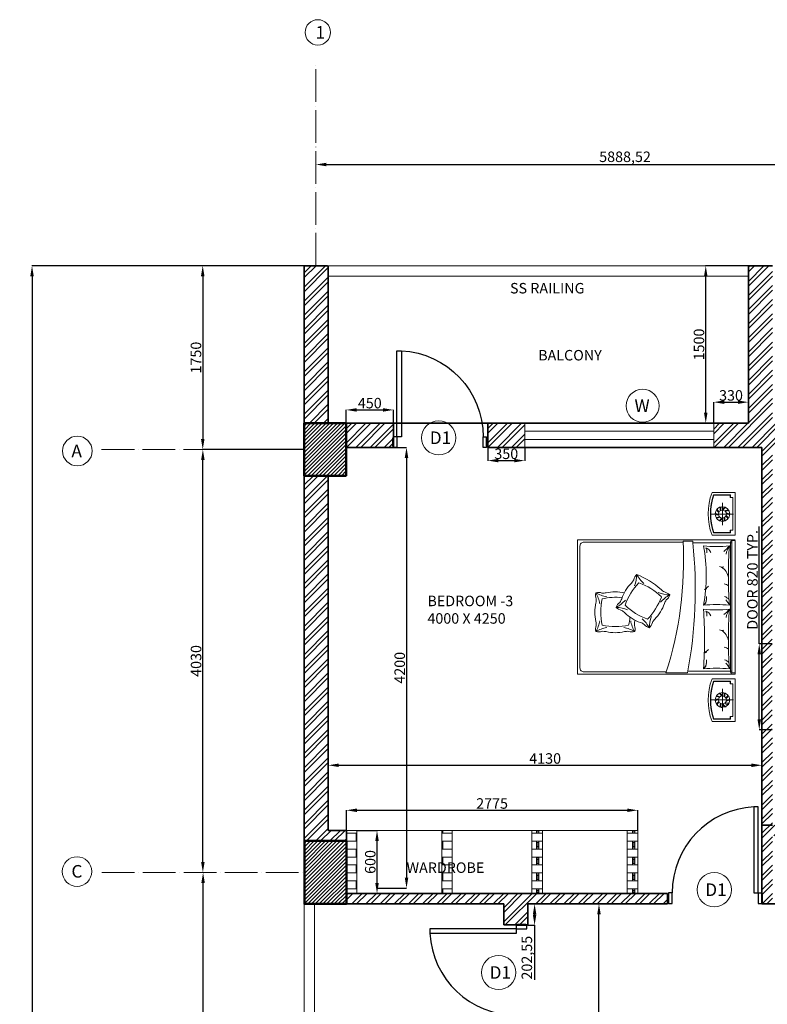
# Model space of a CAD drawing. Units: millimetres. Extents: x -3326 to 29338, y -16792 to 6002.
# Tile 8 of 21: x -3326 to 3793, y -3440 to 5940. Entities that reach past the tile are written whole.
import ezdxf

# ---------------------------------------------------------------- set-up
doc = ezdxf.new("R2010")
doc.units = ezdxf.units.MM
doc.header["$PDMODE"] = 35
doc.header["$PDSIZE"] = 5
doc.linetypes.add('ACAD_ISO04W100', pattern=[30, 24, -3, 0, -3])
for name, color, linetype, lineweight in [('A-ANNO-DIMS', 2, 'Continuous', 13), ('A-ANNO-SYMB', 7, 'Continuous', 18), ('A-AREA-IDEN', 7, 'Continuous', 18), ('A-COLS', 1, 'Continuous', 50), ('A-COLS-PATT', 251, 'Continuous', 13), ('A-DOOR', 3, 'Continuous', 25), ('A-FLOR-CASE', 30, 'Continuous', 18), ('A-FLOR-CASE-PATT', 252, 'Continuous', 13), ('A-FLOR-RAIL', 8, 'Continuous', 20), ('A-GLAZ', 4, 'Continuous', 18), ('A-GRID', 8, 'ACAD_ISO04W100', 13), ('A-GRID-IDEN', 7, 'Continuous', 18), ('A-WALL', 7, 'Continuous', 35), ('A-WALL-PATT', 252, 'Continuous', 13), ('furn', 28, 'Continuous', 18), ('txt', 7, 'Continuous', 18)]:
    doc.layers.add(name, color=color, linetype=linetype, lineweight=lineweight)
doc.styles.get("Standard").update_dxf_attribs({"font": 'arial.ttf'})
doc.dimstyles.new('ISO-25', dxfattribs={"dimtxt": 100, "dimasz": 100, "dimexe": 1.25, "dimexo": 0.625, "dimtad": 1, "dimtxsty": 'Standard', "dimcen": 2.5, "dimadec": 0, "dimazin": 0, "dimtfac": 1, "dimtmove": 0, "dimatfit": 3, "dimfxl": 1, "dimarcsym": 0})

# ---------------------------------------------------------------- blocks, each defined once
blk = doc.blocks.new('A$C0CE462CD')
for p, q in [((860, 100), (860, 0)), ((860, 0), (893.9, 0))]:
    blk.add_line(p, q)
for points in [[(860, 100), (860, 920), (818.4, 920), (818.4, 100)], [(0, 10), (6.1, 10), (6.1, 90), (0, 90)], [(893.9, 10), (900, 10), (900, 90), (893.9, 90)]]:
    blk.add_lwpolyline(points, close=True)
for points in [[(6.1, 0), (40, 0), (40, 100), (6.1, 100)], [(6.1, 100), (6.1, 0)], [(860, 100), (893.9, 100), (893.9, 0)]]:
    blk.add_lwpolyline(points)
blk.add_arc((859.1, 101.9), 819.1, 92.8508, 180.13091)
blk = doc.blocks.new('*D89')
at = {"layer": 'A-ANNO-DIMS', "color": 0, "lineweight": -2, "transparency": 16777216}
for p, q in [((1512.9, -2484), (1578.1, -2484)), ((1576.9, -2584), (1576.9, -2586.5)), ((1512.9, -2686.5), (1578.1, -2686.5)), ((1576.9, -2686.5), (1576.9, -3205.3))]:
    blk.add_line(p, q, dxfattribs=at)
at = {"layer": 'A-ANNO-DIMS', "color": 0, "transparency": 16777216}
for points in [[(1560.2, -2584), (1593.5, -2584), (1576.9, -2484)], [(1560.2, -2586.5), (1593.5, -2586.5), (1576.9, -2686.5)]]:
    blk.add_solid(points, dxfattribs=at)
at = {"layer": 'Defpoints', "color": 0, "transparency": 16777216}
for p in [(1512.3, -2484), (1512.3, -2686.5), (1576.9, -2686.5)]:
    blk.add_point(p, dxfattribs=at)
at = {"layer": 'A-ANNO-DIMS', "color": 0, "transparency": 16777216, "insert": (1516.1, -2995.9), "char_height": 100, "attachment_point": 5, "rotation": 90}
blk.add_mtext('202,55', dxfattribs=at)
blk = doc.blocks.new('*D90')
at = {"layer": 'A-ANNO-DIMS', "color": 0, "lineweight": -2, "transparency": 16777216}
for p, q in [((2190.5, -2484), (2191.1, -2484)), ((2189.9, -6350.4), (2189.9, -2584)), ((2190.5, -6450.4), (2191.1, -6450.4))]:
    blk.add_line(p, q, dxfattribs=at)
at = {"layer": 'A-ANNO-DIMS', "color": 0, "transparency": 16777216}
for points in [[(2173.2, -2584), (2206.5, -2584), (2189.9, -2484)], [(2173.2, -6350.4), (2206.5, -6350.4), (2189.9, -6450.4)]]:
    blk.add_solid(points, dxfattribs=at)
at = {"layer": 'Defpoints', "color": 0, "transparency": 16777216}
for p in [(2189.9, -2484), (2189.9, -2484), (2189.9, -6450.4)]:
    blk.add_point(p, dxfattribs=at)
at = {"layer": 'A-ANNO-DIMS', "color": 0, "transparency": 16777216, "insert": (2129.1, -4467.2), "char_height": 100, "attachment_point": 5, "rotation": 90}
blk.add_mtext('3966,45', dxfattribs=at)
blk = doc.blocks.new('*D136')
at = {"layer": 'A-ANNO-DIMS', "color": 0, "lineweight": -2, "transparency": 16777216}
for p, q in [((-215.5, -1783.3), (-215.5, -1590.2)), ((-115.5, -1591.5), (2459.5, -1591.5)), ((2559.5, -1783.3), (2559.5, -1590.2))]:
    blk.add_line(p, q, dxfattribs=at)
at = {"layer": 'A-ANNO-DIMS', "color": 0, "transparency": 16777216}
for points in [[(-115.5, -1574.8), (-115.5, -1608.1), (-215.5, -1591.5)], [(2459.5, -1574.8), (2459.5, -1608.1), (2559.5, -1591.5)]]:
    blk.add_solid(points, dxfattribs=at)
at = {"layer": 'Defpoints', "color": 0, "transparency": 16777216}
for p in [(2559.5, -1591.5), (-215.5, -1784), (2559.5, -1784)]:
    blk.add_point(p, dxfattribs=at)
at = {"layer": 'A-ANNO-DIMS', "color": 0, "transparency": 16777216, "insert": (1172, -1539.8), "char_height": 100, "attachment_point": 5}
blk.add_mtext('2775', dxfattribs=at)
blk = doc.blocks.new('*D137')
at = {"layer": 'A-ANNO-DIMS', "color": 0, "lineweight": -2, "transparency": 16777216}
for p, q in [((-114.9, -1784), (77.7, -1784)), ((76.4, -2284), (76.4, -1884)), ((-114.9, -2384), (77.7, -2384))]:
    blk.add_line(p, q, dxfattribs=at)
at = {"layer": 'A-ANNO-DIMS', "color": 0, "transparency": 16777216}
for points in [[(59.7, -1884), (93.1, -1884), (76.4, -1784)], [(59.7, -2284), (93.1, -2284), (76.4, -2384)]]:
    blk.add_solid(points, dxfattribs=at)
at = {"layer": 'Defpoints', "color": 0, "transparency": 16777216}
for p in [(-115.5, -1784), (76.4, -1784), (-115.5, -2384)]:
    blk.add_point(p, dxfattribs=at)
at = {"layer": 'A-ANNO-DIMS', "color": 0, "transparency": 16777216, "insert": (24.7, -2084), "char_height": 100, "attachment_point": 5, "rotation": 90}
blk.add_mtext('600', dxfattribs=at)
blk = doc.blocks.new('*D138')
at = {"layer": 'A-ANNO-DIMS', "color": 0, "lineweight": -2, "transparency": 16777216}
for p, q in [((-387.7, -1162.1), (-387.7, -1161.5)), ((-287.7, -1162.7), (3642.3, -1162.7)), ((3742.3, -1162.1), (3742.3, -1161.5))]:
    blk.add_line(p, q, dxfattribs=at)
at = {"layer": 'A-ANNO-DIMS', "color": 0, "transparency": 16777216}
for points in [[(-287.7, -1146.1), (-287.7, -1179.4), (-387.7, -1162.7)], [(3642.3, -1146.1), (3642.3, -1179.4), (3742.3, -1162.7)]]:
    blk.add_solid(points, dxfattribs=at)
at = {"layer": 'Defpoints', "color": 0, "transparency": 16777216}
for p in [(-387.7, -1162.7), (3742.3, -1162.7), (3742.3, -1162.7)]:
    blk.add_point(p, dxfattribs=at)
at = {"layer": 'A-ANNO-DIMS', "color": 0, "transparency": 16777216, "insert": (1677.3, -1111), "char_height": 100, "attachment_point": 5}
blk.add_mtext('4130', dxfattribs=at)
blk = doc.blocks.new('*D139')
at = {"layer": 'A-ANNO-DIMS', "color": 0, "lineweight": -2, "transparency": 16777216}
for p, q in [((7.9, 1866), (358.4, 1866)), ((357.1, 1766), (357.1, -2234)), ((85.4, -2334), (358.4, -2334))]:
    blk.add_line(p, q, dxfattribs=at)
at = {"layer": 'A-ANNO-DIMS', "color": 0, "transparency": 16777216}
for points in [[(340.5, 1766), (373.8, 1766), (357.1, 1866)], [(340.5, -2234), (373.8, -2234), (357.1, -2334)]]:
    blk.add_solid(points, dxfattribs=at)
at = {"layer": 'Defpoints', "color": 0, "transparency": 16777216}
for p in [(7.3, 1866), (84.7, -2334), (357.1, -2334)]:
    blk.add_point(p, dxfattribs=at)
at = {"layer": 'A-ANNO-DIMS', "color": 0, "transparency": 16777216, "insert": (305.4, -234), "char_height": 100, "attachment_point": 5, "rotation": 90}
blk.add_mtext('4200', dxfattribs=at)
blk = doc.blocks.new('*D140')
at = {"layer": 'A-ANNO-DIMS', "color": 0, "lineweight": -2, "transparency": 16777216}
for p, q in [((-217.7, 2096.7), (-217.7, 2223.8)), ((-117.7, 2222.6), (132.3, 2222.6)), ((232.3, 2096.7), (232.3, 2223.8))]:
    blk.add_line(p, q, dxfattribs=at)
at = {"layer": 'A-ANNO-DIMS', "color": 0, "transparency": 16777216}
for points in [[(-117.7, 2239.2), (-117.7, 2205.9), (-217.7, 2222.6)], [(132.3, 2239.2), (132.3, 2205.9), (232.3, 2222.6)]]:
    blk.add_solid(points, dxfattribs=at)
at = {"layer": 'Defpoints', "color": 0, "transparency": 16777216}
for p in [(232.3, 2222.6), (-217.7, 2096), (232.3, 2096)]:
    blk.add_point(p, dxfattribs=at)
at = {"layer": 'A-ANNO-DIMS', "color": 0, "transparency": 16777216, "insert": (7.3, 2274.3), "char_height": 100, "attachment_point": 5}
blk.add_mtext('450', dxfattribs=at)
blk = doc.blocks.new('*D141')
at = {"layer": 'A-ANNO-DIMS', "color": 0, "lineweight": -2, "transparency": 16777216}
for p, q in [((1132.3, 1865.4), (1132.3, 1738.6)), ((1482.3, 1865.4), (1482.3, 1738.6)), ((1232.3, 1739.9), (1382.3, 1739.9))]:
    blk.add_line(p, q, dxfattribs=at)
at = {"layer": 'A-ANNO-DIMS', "color": 0, "transparency": 16777216}
for points in [[(1232.3, 1756.5), (1232.3, 1723.2), (1132.3, 1739.9)], [(1382.3, 1756.5), (1382.3, 1723.2), (1482.3, 1739.9)]]:
    blk.add_solid(points, dxfattribs=at)
at = {"layer": 'Defpoints', "color": 0, "transparency": 16777216}
for p in [(1132.3, 1866), (1482.3, 1866), (1482.3, 1739.9)]:
    blk.add_point(p, dxfattribs=at)
at = {"layer": 'A-ANNO-DIMS', "color": 0, "transparency": 16777216, "insert": (1307.3, 1791.6), "char_height": 100, "attachment_point": 5}
blk.add_mtext('350', dxfattribs=at)
blk = doc.blocks.new('*D142')
at = {"layer": 'A-ANNO-DIMS', "color": 0, "lineweight": -2, "transparency": 16777216}
for p, q in [((3282.3, 2096.7), (3282.3, 2297.5)), ((3382.3, 2296.3), (3512.3, 2296.3)), ((3612.3, 2096.7), (3612.3, 2297.5))]:
    blk.add_line(p, q, dxfattribs=at)
at = {"layer": 'A-ANNO-DIMS', "color": 0, "transparency": 16777216}
for points in [[(3382.3, 2312.9), (3382.3, 2279.6), (3282.3, 2296.3)], [(3512.3, 2312.9), (3512.3, 2279.6), (3612.3, 2296.3)]]:
    blk.add_solid(points, dxfattribs=at)
at = {"layer": 'Defpoints', "color": 0, "transparency": 16777216}
for p in [(3612.3, 2296.3), (3282.3, 2096), (3612.3, 2096)]:
    blk.add_point(p, dxfattribs=at)
at = {"layer": 'A-ANNO-DIMS', "color": 0, "transparency": 16777216, "insert": (3447.3, 2348), "char_height": 100, "attachment_point": 5}
blk.add_mtext('330', dxfattribs=at)
blk = doc.blocks.new('*D143')
at = {"layer": 'A-ANNO-DIMS', "color": 0, "lineweight": -2, "transparency": 16777216}
for p, q in [((3611.7, 3596), (3205.5, 3596)), ((3206.8, 2196), (3206.8, 3496)), ((3611.7, 2096), (3205.5, 2096))]:
    blk.add_line(p, q, dxfattribs=at)
at = {"layer": 'A-ANNO-DIMS', "color": 0, "transparency": 16777216}
for points in [[(3190.1, 3496), (3223.4, 3496), (3206.8, 3596)], [(3190.1, 2196), (3223.4, 2196), (3206.8, 2096)]]:
    blk.add_solid(points, dxfattribs=at)
at = {"layer": 'Defpoints', "color": 0, "transparency": 16777216}
for p in [(3206.8, 3596), (3612.3, 3596), (3612.3, 2096)]:
    blk.add_point(p, dxfattribs=at)
at = {"layer": 'A-ANNO-DIMS', "color": 0, "transparency": 16777216, "insert": (3155.1, 2846), "char_height": 100, "attachment_point": 5, "rotation": 90}
blk.add_mtext('1500', dxfattribs=at)
blk = doc.blocks.new('*D152')
at = {"layer": 'A-ANNO-DIMS', "color": 0, "lineweight": -2, "transparency": 16777216}
for p, q in [((-506.2, 4561.1), (-506.2, 4561.8)), ((-406.2, 4560.5), (5282.3, 4560.5)), ((5382.3, 4561.1), (5382.3, 4561.8))]:
    blk.add_line(p, q, dxfattribs=at)
at = {"layer": 'A-ANNO-DIMS', "color": 0, "transparency": 16777216}
for points in [[(-406.2, 4577.2), (-406.2, 4543.8), (-506.2, 4560.5)], [(5282.3, 4577.2), (5282.3, 4543.8), (5382.3, 4560.5)]]:
    blk.add_solid(points, dxfattribs=at)
at = {"layer": 'Defpoints', "color": 0, "transparency": 16777216}
for p in [(-506.2, 4560.5), (5382.3, 4560.5), (5382.3, 4560.5)]:
    blk.add_point(p, dxfattribs=at)
at = {"layer": 'A-ANNO-DIMS', "color": 0, "transparency": 16777216, "insert": (2438, 4621.2), "char_height": 100, "attachment_point": 5}
blk.add_mtext('5888,52', dxfattribs=at)
blk = doc.blocks.new('*D164')
at = {"layer": 'A-ANNO-DIMS', "color": 0, "lineweight": -2, "transparency": 16777216}
for p, q in [((-1580.6, -2184), (-1581.2, -2184)), ((-1580, -6694.2), (-1580, -2284)), ((-1581.5, -6794.2), (-1578.7, -6794.2))]:
    blk.add_line(p, q, dxfattribs=at)
at = {"layer": 'A-ANNO-DIMS', "color": 0, "transparency": 16777216}
for points in [[(-1596.7, -2284), (-1563.3, -2284), (-1580, -2184)], [(-1596.7, -6694.2), (-1563.3, -6694.2), (-1580, -6794.2)]]:
    blk.add_solid(points, dxfattribs=at)
at = {"layer": 'Defpoints', "color": 0, "transparency": 16777216}
for p in [(-1580, -2184), (-1580, -2184), (-1582.2, -6794.2)]:
    blk.add_point(p, dxfattribs=at)
at = {"layer": 'A-ANNO-DIMS', "color": 0, "transparency": 16777216, "insert": (-1640.7, -4489.1), "char_height": 100, "attachment_point": 5, "rotation": 90}
blk.add_mtext('4610,23', dxfattribs=at)
blk = doc.blocks.new('*D165')
at = {"layer": 'A-ANNO-DIMS', "color": 0, "lineweight": -2, "transparency": 16777216}
for p, q in [((-1580.6, 1846), (-1583.4, 1846)), ((-1582.2, -2084), (-1582.2, 1746)), ((-1580.6, -2184), (-1583.4, -2184))]:
    blk.add_line(p, q, dxfattribs=at)
at = {"layer": 'A-ANNO-DIMS', "color": 0, "transparency": 16777216}
for points in [[(-1598.8, 1746), (-1565.5, 1746), (-1582.2, 1846)], [(-1598.8, -2084), (-1565.5, -2084), (-1582.2, -2184)]]:
    blk.add_solid(points, dxfattribs=at)
at = {"layer": 'Defpoints', "color": 0, "transparency": 16777216}
for p in [(-1582.2, 1846), (-1580, 1846), (-1580, -2184)]:
    blk.add_point(p, dxfattribs=at)
at = {"layer": 'A-ANNO-DIMS', "color": 0, "transparency": 16777216, "insert": (-1633.9, -169), "char_height": 100, "attachment_point": 5, "rotation": 90}
blk.add_mtext('4030', dxfattribs=at)
blk = doc.blocks.new('*D166')
at = {"layer": 'A-ANNO-DIMS', "color": 0, "lineweight": -2, "transparency": 16777216}
for p, q in [((-618.3, 3596), (-1584.7, 3596)), ((-1583.4, 3496), (-1583.4, 1946)), ((-618.3, 1846), (-1584.7, 1846))]:
    blk.add_line(p, q, dxfattribs=at)
at = {"layer": 'A-ANNO-DIMS', "color": 0, "transparency": 16777216}
for points in [[(-1600.1, 3496), (-1566.7, 3496), (-1583.4, 3596)], [(-1600.1, 1946), (-1566.7, 1946), (-1583.4, 1846)]]:
    blk.add_solid(points, dxfattribs=at)
at = {"layer": 'Defpoints', "color": 0, "transparency": 16777216}
for p in [(-617.7, 3596), (-1583.4, 1846), (-617.7, 1846)]:
    blk.add_point(p, dxfattribs=at)
at = {"layer": 'A-ANNO-DIMS', "color": 0, "transparency": 16777216, "insert": (-1635.1, 2721), "char_height": 100, "attachment_point": 5, "rotation": 90}
blk.add_mtext('1750', dxfattribs=at)
blk = doc.blocks.new('*D167')
at = {"layer": 'A-ANNO-DIMS', "color": 0, "lineweight": -2, "transparency": 16777216}
for p, q in [((-618.3, 3596), (-3210.3, 3596)), ((-3209, 3496), (-3209, -12664)), ((-618.3, -12764), (-3210.3, -12764))]:
    blk.add_line(p, q, dxfattribs=at)
at = {"layer": 'A-ANNO-DIMS', "color": 0, "transparency": 16777216}
for points in [[(-3225.7, 3496), (-3192.4, 3496), (-3209, 3596)], [(-3225.7, -12664), (-3192.4, -12664), (-3209, -12764)]]:
    blk.add_solid(points, dxfattribs=at)
at = {"layer": 'Defpoints', "color": 0, "transparency": 16777216}
for p in [(-617.7, 3596), (-3209, -12764), (-617.7, -12764)]:
    blk.add_point(p, dxfattribs=at)
at = {"layer": 'A-ANNO-DIMS', "color": 0, "transparency": 16777216, "insert": (-3260.8, -4584), "char_height": 100, "attachment_point": 5, "rotation": 90}
blk.add_mtext('16360', dxfattribs=at)
blk = doc.blocks.new('BED-WITH-NIGHTSTANDS')
for p, q in [((1378.9, 2083.2), (1378.9, 1869.8)), ((1272.3, 1976.5), (1485.6, 1976.5)), ((1466.8, 1702.3), (1097.4, 1702.3)), ((1455.8, 1708.6), (1455.8, 473.4)), ((1466.8, 480.5), (1049.3, 480.5)), ((1378.9, 98.8), (1378.9, 312.2)), ((1272.2, 205.5), (1485.6, 205.5))]:
    blk.add_line(p, q)
for points in [[(1279.5, 2182), (1501.4, 2182), (1501.4, 1775.2), (1279.5, 1775.2, -0.181818)], [(1097.4, 1719.6), (1097.4, 1702.3, -0.072944), (1045.8, 463.1), (840.6, 463.1, 0.092568), (1003.3, 1719.6)], [(1198.4, 1674.1, 0.058596), (1445.6, 1674.1, 0.036889), (1445.6, 1107.7, 0.052163), (1198.4, 1107.7, 0.093111)], [(1198.4, 1070.9, 0.058596), (1445.6, 1070.9, 0.036648), (1445.6, 500.8, 0.052163), (1198.4, 500.8, 0.036967)], [(1279.6, 0), (1501.5, 0), (1501.5, 406.8), (1279.6, 406.8, 0.181818)]]:
    blk.add_lwpolyline(points, format="xyb", close=True)
for points in [[(1454.8, 1797.4), (1295, 1797.4, -0.167087), (1295, 2159.8), (1454.8, 2159.8)], [(1454.8, 1799.6), (1296.6, 1799.6, -0.165559), (1296.6, 2157.6), (1454.8, 2157.6)], [(1003.9, 1708.6), (59.2, 1708.6, 0.414214), (22.2, 1671.6), (22.2, 510.4, 0.414214), (59.2, 473.4), (844.2, 473.4)], [(583.2, 1320, 0.111006), (451.8, 1108.7, 0.119549), (665.6, 975.5, 0.107813), (797.5, 1186.1)], [(540, 1293.1, 0.091296), (562.8, 1401.4, 0.091296), (630.7, 1314.1, 0.091296)], [(797.2, 1187.3, 0.121865), (583.2, 1319.9, 0.121865)], [(211.2, 1122.2, 0.091296), (173.3, 1226.2, 0.091296), (277.2, 1187.9, 0.091296)], [(768.3, 1228.3, 0.091296), (876.7, 1205.8, 0.091296), (789.5, 1137.6, 0.091296)], [(233.7, 1167.8, 0.111006), (234, 919, 0.119549), (485.8, 919, 0.033212), (497.4, 995.5)], [(475.6, 1065.1, 0.091296), (367.2, 1087.5, 0.091296), (454.4, 1155.8)], [(367.2, 1087.5, 0.159461), (418, 1058.9, -0.076283), (449.6, 1036.2, 0.115075), (598.7, 943.3, -0.076283), (633, 924.9, 0.159461), (681.1, 892)], [(277.2, 894.6, 0.091296), (173.3, 856.3, 0.091296), (211.2, 960.3)], [(505.3, 960.3, 0.091296), (543.2, 856.3, 0.091296), (439.3, 894.6, 0.091296)], [(703.9, 1000.2, 0.091296), (681.1, 892, 0.091296), (613.2, 979.3, 0.091296)], [(173.3, 856.3, 0.159461), (231.6, 858.9, -0.076283), (270.5, 856.3, 0.115075), (446, 856.3, -0.076283), (484.9, 858.9, 0.159461), (543.2, 856.3)], [(1454.9, 384.6), (1295.1, 384.6, 0.167087), (1295.1, 22.2), (1454.9, 22.2)], [(1454.9, 382.4), (1296.7, 382.4, 0.165559), (1296.7, 24.4), (1454.9, 24.4)]]:
    blk.add_lwpolyline(points, format="xyb")
for points in [[(1479.2, 2133.2), (1452.6, 2133.2), (1452.6, 2159.8)], [(1479.2, 2135.4), (1454.8, 2135.4), (1454.8, 2159.8)], [(1477, 2135.4), (1477, 1821.8)], [(1479.2, 2135.4), (1479.2, 1821.8)], [(1479.2, 1824), (1452.6, 1824), (1452.6, 1797.4)], [(1479.2, 1821.8), (1454.8, 1821.8), (1454.8, 1797.4)], [(1501.5, 1730.8), (0, 1730.8), (0, 451.2), (1501.5, 451.2)], [(1501.5, 463.1), (1466.8, 463.1), (1466.8, 1723.4), (1501.5, 1723.4), (1501.5, 451.2)], [(1479.3, 358), (1452.7, 358), (1452.7, 384.6)], [(1479.3, 360.2), (1454.9, 360.2), (1454.9, 384.6)], [(1477.1, 46.6), (1477.1, 360.2)], [(1479.3, 46.6), (1479.3, 360.2)], [(1479.3, 48.8), (1452.7, 48.8), (1452.7, 22.2)], [(1479.3, 46.6), (1454.9, 46.6), (1454.9, 22.2)]]:
    blk.add_lwpolyline(points)
for centre, radius in [((1378.9, 1976.5), 69.7), ((1378.9, 1976.5), 37.8), ((1378.9, 205.5), 69.7), ((1378.9, 205.5), 37.8)]:
    blk.add_circle(centre, radius)
for centre, radius, start, end in [((1340.3, 2012.2), 44.8, 226.17003, 272.48975), ((1338.5, 2008.1), 34.1, 214.30017, 274.53802), ((1368.7, 2028), 44.8, 190.17003, 236.48975), ((1364.8, 2025.8), 34.1, 178.30017, 238.53802), ((1400.9, 2024.2), 44.8, 154.17003, 200.48975), ((1396.5, 2024.6), 34.1, 142.30017, 202.53802), ((1424.8, 2002.2), 44.8, 118.17003, 164.48975), ((1421.4, 2005.1), 34.1, 106.30017, 166.53802), ((1431.1, 1970.3), 44.8, 82.17003, 128.48975), ((1430.1, 1974.7), 34.1, 70.30017, 130.53802), ((1417.5, 1940.8), 44.8, 46.17003, 92.48975), ((1419.3, 1944.9), 34.1, 34.30017, 94.53802), ((1327.7, 1978.3), 34.1, 250.30017, 310.53802), ((1326.7, 1982.7), 44.8, 262.17003, 308.48975), ((1336.4, 1947.9), 34.1, 286.30017, 346.53802), ((1333.1, 1950.8), 44.8, 298.17003, 344.48975), ((1361.4, 1928.3), 34.1, 322.30017, 22.53802), ((1356.9, 1928.8), 44.8, 334.17003, 20.48975), ((1393, 1927.2), 34.1, 358.30017, 58.53802), ((1389.2, 1925), 44.8, 10.17003, 56.48975), ((1478, 1708.6), 22.2, 90, 180), ((1175.6, 1619.4), 56.2, 346.48229, 38.55627), ((1192.7, 1576.7), 82.2, 24.2916, 70.9896), ((1214.5, 1859.4), 296.3, 306.49353, 321.27919), ((1652.3, 1542.6), 244.9, 147.53791, 167.5233), ((1375.3, 1532.7), 61.4, 245.89274, 286.11919), ((1299.1, 1354.7), 137.1, 6.68493, 58.3182), ((785.6, 1046.2), 386.5, 135.13065, 161.38844), ((419.7, 1408.4), 128.4, 315.77185, 333.2208), ((626.3, 1332.5), 93.8, 132.65224, 168.89294), ((256.3, 651.7), 810, 48.38179, 67.76439), ((263.7, 1201.2), 93.8, 164.57915, 200.81985), ((198.5, 1135.9), 93.8, 69.36661, 105.60731), ((242.7, 1351.6), 128.4, 265.03874, 282.4877), ((358.2, 849.8), 386.5, 76.87111, 103.12889), ((884.1, 1348.9), 128.4, 225.58539, 243.03435), ((807.5, 1142.5), 93.8, 42.46578, 78.70648), ((1208.9, 1279), 20.7, 263.75428, 347.21866), ((1026.5, 1507.4), 308.8, 306.20852, 315.08491), ((1377, 1216.1), 96.2, 51.81741, 79.89867), ((550.3, 1042.5), 386.5, 167.05756, 193.31535), ((48.2, 1156.4), 128.4, 347.69876, 5.14771), ((360.8, 659.2), 524.3, 83.19556, 104.02838), ((468.2, 1051.5), 107.3, 128.77541, 160.35713), ((298.1, 1211.9), 128.4, 323.29829, 340.74724), ((947.4, 1081.9), 128.4, 143.29829, 160.74724), ((789.7, 1230.6), 90.5, 307.29372, 344.09733), ((1127.7, 1179.9), 101.1, 314.40604, 6.83423), ((1163, 1161), 64, 303.63488, 0.84559), ((1363.4, 1094.5), 103.5, 40.53543, 70.35581), ((1276.2, 1030), 186.4, 24.64565, 44.15848), ((460, 1247.6), 386.5, 315.13065, 341.38844), ((1175.6, 1016.2), 56.2, 346.48229, 38.55627), ((1192.7, 973.5), 82.2, 24.2916, 70.9896), ((1214.5, 1256.2), 296.3, 306.49353, 321.27919), ((1652.3, 939.4), 244.9, 147.53791, 167.5233), ((48.9, 925.3), 128.4, 355.2252, 12.67415), ((669.5, 927.3), 128.4, 167.69876, 185.14771), ((167.4, 1041.2), 386.5, 347.05756, 348.7033), ((626.1, 958.8), 86.6, 309.47264, 349.6505), ((825.9, 885.4), 128.4, 135.77185, 153.2208), ((278.1, 879.2), 107.3, 160.70232, 192.28404), ((461.1, 884), 86.6, 341.39955, 21.57741), ((1375.3, 929.5), 61.4, 245.89274, 286.11919), ((1299.1, 751.6), 137.1, 6.68493, 58.3182), ((1208.9, 675.8), 20.7, 263.75428, 347.21866), ((1026.5, 904.2), 308.8, 306.20852, 315.08491), ((1377, 612.9), 96.2, 51.81741, 79.89867), ((1127.7, 576.7), 101.1, 314.40604, 6.83423), ((1363.4, 491.3), 103.5, 40.53543, 70.35581), ((1163, 557.8), 64, 303.63488, 0.84559), ((1276.2, 426.8), 186.4, 24.64565, 44.15848), ((1478, 473.4), 22.2, 180, 270), ((1340.3, 169.8), 44.8, 87.51025, 133.82997), ((1338.5, 173.9), 34.1, 85.46198, 145.69983), ((1327.7, 203.7), 34.1, 49.46198, 109.69983), ((1326.7, 199.3), 44.8, 51.51025, 97.82997), ((1368.6, 154), 44.8, 123.51025, 169.82997), ((1336.4, 234.2), 34.1, 13.46198, 73.69983), ((1333, 231.2), 44.8, 15.51025, 61.82997), ((1361.4, 253.7), 34.1, 337.46198, 37.69983), ((1356.9, 253.2), 44.8, 339.51025, 25.82997), ((1393, 254.8), 34.1, 301.46198, 1.69983), ((1389.2, 257.1), 44.8, 303.51025, 349.82997), ((1417.5, 241.2), 44.8, 267.51025, 313.82997), ((1419.3, 237.1), 34.1, 265.46198, 325.69983), ((1364.8, 156.2), 34.1, 121.46198, 181.69983), ((1402.8, 152.7), 44.8, 159.51025, 205.82997), ((1398.4, 152.3), 34.1, 157.46198, 217.69983), ((1426.7, 174.7), 44.8, 195.51025, 241.82997), ((1423.3, 171.8), 34.1, 193.46198, 253.69983), ((1433, 206.6), 44.8, 231.51025, 277.82997), ((1430.1, 207.3), 34.1, 229.46198, 289.69983)]:
    blk.add_arc(centre, radius, start, end)
blk = doc.blocks.new('TAG-D1')
blk.add_circle((163.3, 163.3), 163.3)
at = {"insert": (78, 223.5), "char_height": 120, "attachment_point": 1}
blk.add_mtext_dynamic_manual_height_columns('D1', width=137.943, gutter_width=12.5, heights=[0], dxfattribs=at)
blk = doc.blocks.new('TAG-W')
blk.add_circle((156.8, 156.8), 156.8)
at = {"insert": (79.7, 216.8), "char_height": 120, "attachment_point": 1}
blk.add_mtext_dynamic_manual_height_columns('W', width=376.575, gutter_width=12.5, heights=[0], dxfattribs=at)
blk = doc.blocks.new('GLAZ-1800x80')
for p, q in [((0, 80), (1800, 80)), ((0, 0), (1800, 0))]:
    blk.add_line(p, q)
blk = doc.blocks.new('*D197')
at = {"layer": 'A-ANNO-DIMS', "color": 0, "lineweight": -2, "transparency": 16777216}
for p, q in [((3716.3, -5.8), (3716.3, 1112.9)), ((3838.6, -5.8), (3715, -5.8)), ((3716.3, -725.8), (3716.3, -105.8)), ((3838.6, -825.8), (3715, -825.8))]:
    blk.add_line(p, q, dxfattribs=at)
at = {"layer": 'A-ANNO-DIMS', "color": 0, "transparency": 16777216}
for points in [[(3699.6, -105.8), (3732.9, -105.8), (3716.3, -5.8)], [(3699.6, -725.8), (3732.9, -725.8), (3716.3, -825.8)]]:
    blk.add_solid(points, dxfattribs=at)
at = {"layer": 'Defpoints', "color": 0, "transparency": 16777216}
for p in [(3716.3, -5.8), (3839.3, -5.8), (3839.3, -825.8)]:
    blk.add_point(p, dxfattribs=at)
at = {"layer": 'A-ANNO-DIMS', "color": 0, "transparency": 16777216, "insert": (3663.9, 603.5), "char_height": 100, "attachment_point": 5, "rotation": 90}
blk.add_mtext('DOOR 820 TYP.', dxfattribs=at)

msp = doc.modelspace()

# ---------------------------------------------------------------- hatches: boundary and pattern name
at = {"layer": 'A-COLS-PATT'}
h = msp.add_hatch(dxfattribs=at)
h.set_pattern_fill('ANSI31', color=256, scale=8)
h.set_pattern_definition([(45, (-45233.41, 7309.686), (-17.960512, 17.960512), [])])
h.paths.add_polyline_path([(-617.699, 2096.048), (-617.699, 1596.048), (-217.699, 1596.048), (-217.699, 2096.048)])
h = msp.add_hatch(dxfattribs=at)
h.set_pattern_fill('ANSI31', color=256, scale=8)
h.set_pattern_definition([(45, (-42336.819, 4723.052), (-17.960512, 17.960512), [])])
h.paths.add_polyline_path([(-615.519, -2483.952), (-215.519, -2483.952), (-215.519, -1883.952), (-615.519, -1883.952)])
at = {"layer": 'A-FLOR-CASE-PATT'}
h = msp.add_hatch(dxfattribs=at)
h.set_pattern_fill('BRSTONE', color=256, scale=9)
h.set_pattern_definition([(0, (-10476.645, 1e-12), (0, 75.438), []), (90, (-10270.9, 1e-12), (-114.3, 75.438), [75.438, -75.438]), (90, (-10293.77, 1e-12), (-114.3, 75.438), [75.438, -75.438]), (0, (-10270.905, 12.57), (114.3, 75.438), [-205.74, 22.86]), (0, (-10270.905, 25.146), (114.3, 75.438), [-205.74, 22.86]), (0, (-10270.905, 37.72), (114.3, 75.438), [-205.74, 22.86]), (0, (-10270.905, 50.29), (114.3, 75.438), [-205.74, 22.86]), (0, (-10270.905, 62.865), (114.3, 75.438), [-205.74, 22.86])])
h.paths.add_polyline_path([(-115.519, -1783.952), (-215.519, -1783.952), (-215.519, -1883.952), (-215.519, -2383.952), (-115.519, -2383.952)])
h.paths.add_polyline_path([(792.814, -1783.952), (692.814, -1783.952), (692.814, -2383.952), (792.814, -2383.952)])
h.paths.add_polyline_path([(1651.147, -1783.952), (1551.147, -1783.952), (1551.147, -2383.952), (1651.147, -2383.952)])
h.paths.add_polyline_path([(2559.481, -1783.952), (2459.481, -1783.952), (2459.481, -2383.952), (2559.481, -2383.952)])
at = {"layer": 'A-WALL-PATT'}
h = msp.add_hatch(dxfattribs=at)
h.set_pattern_fill('ANSI32', color=256, scale=10)
h.set_pattern_definition([(45, (-10476.65, 1e-12), (-67.3519, 67.3519), []), (45, (-10431.74, 1e-12), (-67.3519, 67.3519), [])])
h.paths.add_polyline_path([(2842.301, -2383.952), (-215.519, -2383.952), (-215.519, -2483.952), (1282.301, -2483.952), (1282.301, -2683.952), (1413.549, -2683.952), (1413.549, -2680.395), (1493.875, -2680.395), (1512.301, -2683.952), (1512.301, -2483.952), (2842.301, -2483.952)])
h.paths.add_polyline_path([(1512.301, -3583.952), (1493.875, -3583.952), (1493.875, -3584.058), (1413.549, -3584.058), (1282.301, -3583.952), (1282.301, -4183.952), (1512.301, -4183.952)])
h.paths.add_polyline_path([(5172.301, -1733.952), (3842.301, -1733.952), (3742.301, -1733.952), (3742.301, -1833.952), (3742.301, -2389.299), (3746.327, -2389.299), (3746.327, -2469.299), (3742.301, -2469.299), (3742.301, -2483.952), (3842.301, -2483.952), (3842.301, -1833.952), (5172.301, -1833.952)])
h.paths.add_polyline_path([(5572.301, 1346.048), (5342.301, 1346.048), (5342.301, -733.952), (4642.301, -733.952), (4642.301, -833.952), (5342.301, -833.952), (5342.301, -1733.952), (5572.301, -1733.952), (5572.301, -1033.952), (6402.301, -1033.952), (6402.301, -933.952), (5572.301, -933.952)])
h.paths.add_polyline_path([(4092.301, 2096.048), (3842.301, 2096.048), (3842.301, 3596.048), (3612.301, 3596.048), (3612.301, 2096.048), (3282.301, 2096.048), (3282.301, 1866.048), (3612.301, 1866.048), (3742.301, 1866.048), (3742.301, -1733.952), (3842.301, -1733.952), (3842.301, -815.784), (3839.26, -815.784), (3839.26, -735.784), (3842.301, 1866.048), (4092.301, 1866.048)])
h.paths.add_polyline_path([(7302.301, 3596.048), (7072.301, 3596.048), (7072.301, 2096.048), (6672.301, 2096.048), (6672.301, 1866.048), (7202.301, 1866.048), (7202.301, -943.25), (7207.296, -943.25), (7207.296, -1023.25), (7202.301, -1033.952), (7217.026, -1033.952), (7217.026, -1030.415), (7302.301, -1030.415), (7302.301, 1866.048), (7302.301, 1946.048)])
h.paths.add_polyline_path([(6072.301, 2096.048), (5572.301, 2096.048), (5572.301, 1866.048), (6072.301, 1866.048)])
h.paths.add_polyline_path([(5172.301, 2096.048), (4692.301, 2096.048), (4692.301, 1866.048), (5172.301, 1866.048)])
h.paths.add_polyline_path([(4792.301, 2496.048), (4692.301, 2496.048), (4692.301, 2096.048), (4792.301, 2096.048)])
h.paths.add_polyline_path([(6072.301, 2496.048), (5972.301, 2496.048), (5972.301, 2096.048), (6072.301, 2096.048)])
h.paths.add_polyline_path([(1482.301, 2096.048), (1132.301, 2096.048), (1132.301, 1866.048), (1482.301, 1866.048)])
h.paths.add_polyline_path([(232.301, 2096.048), (-217.699, 2096.048), (-217.699, 1866.048), (232.301, 1866.048), (232.301, 1876.048), (226.22, 1876.048), (226.22, 1956.048)])
h.paths.add_polyline_path([(-387.699, 3596.048), (-394.734, 3596.048), (-617.699, 3596.048), (-617.699, 2096.048), (-387.699, 2096.048)])
h.paths.add_polyline_path([(-387.699, 1596.048), (-617.699, 1596.048), (-617.699, 336.048), (-617.699, -1883.952), (-215.519, -1883.952), (-215.519, -1783.952), (-387.699, -1783.952)])

# ---------------------------------------------------------------- linework, layer by layer
at = {"layer": 'A-COLS'}
for points in [[(-617.699, 2096.048), (-217.699, 2096.048), (-217.699, 1596.048), (-617.699, 1596.048)], [(-615.519, -1883.952), (-215.519, -1883.952), (-215.519, -2483.952), (-615.519, -2483.952)]]:
    msp.add_lwpolyline(points, close=True, dxfattribs=at)
at = {"layer": 'A-FLOR-CASE'}
for p, q in [((-215.519, -1783.952), (-115.519, -1783.952)), ((-115.519, -1783.952), (-115.519, -2383.952)), ((-115.519, -1783.952), (2459.481, -1783.952)), ((692.814, -1783.952), (692.814, -2383.952)), ((792.814, -1783.952), (792.814, -2383.952)), ((1551.147, -1783.952), (1551.147, -2383.952)), ((1651.147, -1783.952), (1651.147, -2383.952)), ((2459.481, -1783.952), (2459.481, -2383.952)), ((2459.481, -1783.952), (2559.481, -1783.952)), ((2559.481, -1783.952), (2559.481, -2383.952))]:
    msp.add_line(p, q, dxfattribs=at)
at = {"layer": 'A-FLOR-RAIL'}
for p, q in [((3612.301, 3596.048), (-394.734, 3596.048)), ((3612.301, 3496.048), (-394.734, 3496.048)), ((-617.699, -2483.952), (-617.699, -6450.401)), ((-517.699, -2483.952), (-517.699, -6450.401))]:
    msp.add_line(p, q, dxfattribs=at)
at = {"layer": 'A-GLAZ'}
for p, q in [((1482.301, 1866.048), (1482.301, 2096.048)), ((3282.301, 1866.048), (3282.301, 2096.048))]:
    msp.add_line(p, q, dxfattribs=at)
at = {"layer": 'A-GRID', "ltscale": 13}
for p, q in [((-506.217, 3596.048), (-506.217, 5524.981)), ((-2546.632, 1846.048), (-617.699, 1846.048)), ((-2544.452, -2183.952), (-615.519, -2183.952))]:
    msp.add_line(p, q, dxfattribs=at)
at = {"layer": 'A-GRID-IDEN'}
for centre, radius in [((-487.268, 5819.473), 120.678), ((-2777.642, 1831.264), 141.47), ((-2780.629, -2175.171), 140.921)]:
    msp.add_circle(centre, radius, dxfattribs=at)
at = {"layer": 'A-WALL'}
for p, q in [((-617.699, 336.048), (-617.699, 3596.048)), ((-394.734, 3596.048), (-617.699, 3596.048)), ((-387.699, 3596.048), (-387.699, 2096.048)), ((3612.301, 3596.048), (3612.301, 2096.048)), ((3842.301, 3596.048), (3612.301, 3596.048)), ((3612.301, 2096.048), (-387.699, 2096.048)), ((232.301, 1866.048), (232.301, 2096.048)), ((1132.301, 1866.048), (1132.301, 2096.048)), ((232.301, 1866.048), (-217.699, 1866.048)), ((3612.301, 1866.048), (1132.301, 1866.048)), ((3742.301, 1866.048), (3612.301, 1866.048)), ((3742.301, 1866.048), (3742.301, -1733.952)), ((-387.699, 1596.048), (-387.699, -1783.952)), ((-617.699, 336.048), (-617.699, -2483.952)), ((3842.301, -1733.952), (3742.301, -1733.952)), ((3742.301, -1833.952), (3742.301, -1733.952)), ((-215.519, -1783.952), (-387.699, -1783.952)), ((-215.519, -1883.952), (-215.519, -1783.952)), ((3742.301, -1833.952), (3742.301, -2483.952)), ((2842.301, -2383.952), (-215.519, -2383.952)), ((2842.301, -2383.952), (2842.301, -2483.952)), ((-387.699, -2483.952), (-617.699, -2483.952)), ((1282.301, -2483.952), (-387.699, -2483.952)), ((1282.301, -2483.952), (1282.301, -2683.952)), ((2842.301, -2483.952), (1512.301, -2483.952)), ((1512.301, -2483.952), (1512.301, -2683.952)), ((5572.301, -2483.952), (3742.301, -2483.952)), ((1512.301, -2683.952), (1282.301, -2683.952))]:
    msp.add_line(p, q, dxfattribs=at)

# ---------------------------------------------------------------- block references
at = {"layer": 'A-ANNO-SYMB'}
for name, p in [('TAG-W', (2448.742, 2105.323)), ('TAG-D1', (500.809, 1793.582)), ('TAG-D1', (3123.957, -2511.765)), ('TAG-D1', (1070.368, -3300.303))]:
    msp.add_blockref(name, p, dxfattribs=at)
at = {"layer": 'A-DOOR', "xscale": -1}
msp.add_blockref('A$C0CE462CD', (1126.22, 1866.048), dxfattribs=at)
at = {"layer": 'A-DOOR'}
msp.add_blockref('A$C0CE462CD', (2846.327, -2479.299), dxfattribs=at)
at = {"layer": 'A-DOOR', "xscale": 1.004070386304363, "yscale": 1.004070386304363, "zscale": 1.004070386304363, "rotation": 90.00000000000003}
msp.add_blockref('A$C0CE462CD', (1503.915, -3584.058), dxfattribs=at)
at = {"layer": 'A-GLAZ'}
msp.add_blockref('GLAZ-1800x80', (1482.301, 1941.048), dxfattribs=at)
at = {"layer": 'furn'}
msp.add_blockref('BED-WITH-NIGHTSTANDS', (1986.761, -745.907), dxfattribs=at)

# ---------------------------------------------------------------- texts
at = {"layer": 'A-AREA-IDEN', "char_height": 100, "attachment_point": 1}
for s, width, insert in [('BALCONY', 1168.90663, (1610.8, 2793.605)), ('BEDROOM -3\\P4000 X 4250', 1087.98512, (556.114, 452.703))]:
    msp.add_mtext_dynamic_manual_height_columns(s, width=width, gutter_width=12.5, heights=[0], dxfattribs=dict(at, insert=insert))
at = {"layer": 'A-GRID-IDEN', "char_height": 120, "attachment_point": 1}
for s, width, insert in [('1', 463.74815, (-509.369, 5879.718)), ('A', 319.52755, (-2833.672, 1891.264)), ('C', 319.52755, (-2833.672, -2113.125))]:
    msp.add_mtext_dynamic_manual_height_columns(s, width=width, gutter_width=12.5, heights=[0], dxfattribs=dict(at, insert=insert))
at = {"layer": 'txt', "char_height": 100, "attachment_point": 1}
for s, insert in [('SS RAILING', (1342.482, 3432.028)), ('WARDROBE', (357.123, -2088.121))]:
    msp.add_mtext_dynamic_manual_height_columns(s, width=1168.90663, gutter_width=12.5, heights=[0], dxfattribs=dict(at, insert=insert))

# ---------------------------------------------------------------- dimensions: what is measured, and where the dimension line sits
at = {"layer": 'A-ANNO-DIMS'}
for base, p1, p2, picture, middle in [((5382.301, 4560.514), (-506.217, 4560.514), (5382.301, 4560.514), '*D152', (2438.042, 4621.235)), ((3612.301, 2296.268), (3282.301, 2096.048), (3612.301, 2096.048), '*D142', (3447.301, 2347.985)), ((232.301, 2222.579), (-217.699, 2096.048), (232.301, 2096.048), '*D140', (7.301, 2274.261)), ((1482.301, 1739.859), (1132.301, 1866.048), (1482.301, 1866.048), '*D141', (1307.301, 1791.576)), ((3742.301, -1162.744), (-387.699, -1162.744), (3742.301, -1162.744), '*D138', (1677.301, -1111.028)), ((2559.481, -1591.466), (-215.519, -1783.952), (2559.481, -1783.952), '*D136', (1171.981, -1539.784))]:
    dim = msp.add_linear_dim(base=base, p1=p1, p2=p2, dimstyle='ISO-25', override={"dimclrd": 0, "dimclre": 0, "dimclrt": 0}, dxfattribs=at)
    dim.commit()
    dim.dimension.update_dxf_attribs({"geometry": picture, "text_midpoint": middle})
for base, p1, p2, picture, middle in [((-3209.046, -12763.952), (-617.699, 3596.048), (-617.699, -12763.952), '*D167', (-3260.762, -4583.952)), ((-1583.416, 1846.048), (-617.699, 3596.048), (-617.699, 1846.048), '*D166', (-1635.098, 2721.048)), ((3206.756, 3596.048), (3612.301, 2096.048), (3612.301, 3596.048), '*D143', (3155.073, 2846.048)), ((-1582.166, 1846.048), (-1579.986, -2183.952), (-1579.986, 1846.048), '*D165', (-1633.882, -168.952)), ((357.123, -2333.952), (7.301, 1866.048), (84.738, -2333.952), '*D139', (305.441, -233.952)), ((76.405, -1783.952), (-115.519, -2383.952), (-115.519, -1783.952), '*D137', (24.723, -2083.952)), ((-1579.986, -2183.952), (-1582.166, -6794.183), (-1579.986, -2183.952), '*D164', (-1640.706, -4489.067)), ((1576.858, -2686.501), (1512.301, -2483.952), (1512.301, -2686.501), '*D89', (1516.137, -2995.925)), ((2189.865, -2483.952), (2189.865, -6450.401), (2189.865, -2483.952), '*D90', (2129.144, -4467.177))]:
    dim = msp.add_linear_dim(base=base, p1=p1, p2=p2, angle=90, dimstyle='ISO-25', override={"dimclrd": 0, "dimclre": 0, "dimclrt": 0}, dxfattribs=at)
    dim.commit()
    dim.dimension.update_dxf_attribs({"geometry": picture, "text_midpoint": middle})
dim = msp.add_linear_dim(base=(3716.26, -5.784), p1=(3839.26, -825.784), p2=(3839.26, -5.784), angle=90, text='DOOR <> TYP.', dimstyle='ISO-25', override={"dimdec": 0, "dimlfac": 1, "dimrnd": 0, "dimzin": 0, "dimdsep": 46, "dimlunit": 2}, dxfattribs=at)
dim.commit()
dim.dimension.update_dxf_attribs({"geometry": '*D197', "text_midpoint": (3663.896, 603.538)})

doc.saveas('drawing.dxf')
